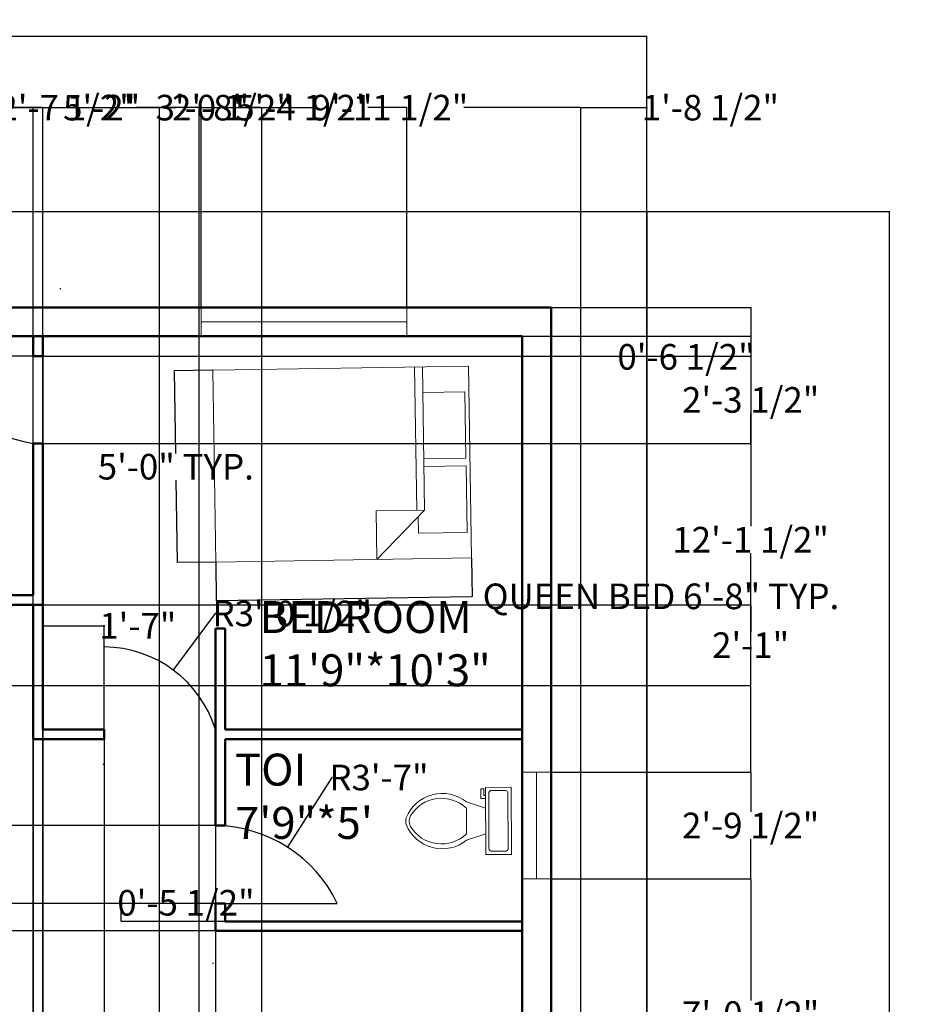
# Model space of a CAD drawing. Units: inches. Extents: x 3437 to 3994, y 3379 to 4084.
# Tile 6 of 6: x 3715 to 3994, y 3776 to 4084. Entities that reach past the tile are written whole.
import ezdxf

# ---------------------------------------------------------------- set-up
doc = ezdxf.new("R2010")
doc.units = ezdxf.units.IN
doc.header["$MEASUREMENT"] = 0
for name, color, linetype, lineweight in [('A-ANNO-DIMS', 2, 'Continuous', 18), ('A-AREA-IDEN', 7, 'Continuous', 25), ('A-DOOR', 3, 'Continuous', 25), ('A-FLOR-FIXT', 9, 'Continuous', 18), ('A-FURN', 8, 'Continuous', 18), ('A-GLAZ', 4, 'Continuous', 18), ('A-WALL', 7, 'Continuous', 50), ('C-PROP', 3, 'Continuous', 25)]:
    doc.layers.add(name, color=color, linetype=linetype, lineweight=lineweight)
doc.styles.get("Standard").update_dxf_attribs({"font": 'arial.ttf'})
doc.dimstyles.get("Standard").update_dxf_attribs({"dimtxt": 8, "dimasz": 0.18, "dimexe": 0.18, "dimexo": 0.0625, "dimgap": 0.09, "dimtad": 0, "dimtih": 1, "dimtoh": 1, "dimdec": 0, "dimzin": 0, "dimdsep": 46, "dimlunit": 3, "dimtxsty": 'Standard', "dimcen": 0.09, "dimadec": 0, "dimazin": 0, "dimtfac": 1, "dimtdec": 0, "dimtofl": 0, "dimtmove": 0, "dimatfit": 3, "dimfxl": 1, "dimtolj": 1, "dimtzin": 0, "dimarcsym": 0})

# ---------------------------------------------------------------- blocks, each defined once
blk = doc.blocks.new('Bed - Queen')
for p, q in [((0, -80.00003), (0, 0)), ((0, 0), (59.99999, 0)), ((59.99999, 0), (59.99999, -80.00003)), ((7.99999, -1.2), (28.79998, -1.2)), ((7.99999, -14.4), (7.99999, -1.2)), ((28.79998, -1.2), (28.79998, -14.4)), ((31.19999, -1.2), (51.99999, -1.2)), ((31.19999, -14.4), (31.19999, -1.2)), ((51.99999, -1.2), (51.99999, -16.4)), ((0, -14.4), (44.8, -14.4)), ((59.99999, -29.6), (44.8, -14.4)), ((44.8, -14.4), (44.8, -29.6)), ((44.8, -16.8), (0, -16.8)), ((51.99999, -16.4), (46.79936, -16.4)), ((44.8, -29.6), (59.99999, -29.6)), ((59.99999, -80.00003), (0, -80.00003))]:
    blk.add_line(p, q)
blk = doc.blocks.new('Toilet - top')
for p, q in [((9.5, -6), (9.5, -2)), ((-10, -8.5), (-8, -8.5)), ((-10, -9.5), (-10, -8.5)), ((-8, -8.5), (-8, -8)), ((-7, -8), (-7, -9.5)), ((-4, -8), (-6, -14)), ((4, -8), (6, -14)), ((-7, -9.5), (-10, -9.5)), ((4, -14), (-4, -14))]:
    blk.add_line(p, q)
blk.add_lwpolyline([(10.5, -8), (10.5, 0), (-10.5, 0), (-10.5, -8)], close=True)
for points in [[(-9.5, -2), (-9.5, -6)], [(8.5, -1), (-8.5, -1)], [(-8.5, -7), (8.5, -7)]]:
    blk.add_lwpolyline(points)
for centre, radius, start, end in [((-8.62, -1.88), 0.884, 81.8699, 188.1301), ((8.62, -1.88), 0.884, 351.8699, 98.1301), ((-8.62, -6.12), 0.884, 171.8699, 278.1301), ((8.62, -6.12), 0.884, 261.8699, 8.1301), ((3.52, -21.58), 12.17, 141.4691, 247.9714), ((4.2, -21.82), 11.33, 136.3677, 238.9468), ((-3.52, -21.58), 12.17, 292.0284, 38.5307), ((-4.2, -21.82), 11.33, 301.053, 43.6321), ((0, -27.88), 4, 245.7318, 294.2682), ((0, -29), 4, 254.8605, 285.1395)]:
    blk.add_arc(centre, radius, start, end)
blk = doc.blocks.new('*D9')
at = {"layer": 'A-ANNO-DIMS', "color": 0, "lineweight": -2, "transparency": 16777216}
for p, q in [((3491.02, 4023.7), (3491.02, 4078.52)), ((3491.2, 4078.34), (3694.15, 4078.34)), ((3910.84, 4078.34), (3707.9, 4078.34)), ((3911.02, 4023.7), (3911.02, 4078.52))]:
    blk.add_line(p, q, dxfattribs=at)
at = {"layer": 'A-ANNO-DIMS', "color": 0, "transparency": 16777216}
for points in [[(3491.2, 4078.37), (3491.2, 4078.31), (3491.02, 4078.34)], [(3910.84, 4078.37), (3910.84, 4078.31), (3911.02, 4078.34)]]:
    blk.add_solid(points, dxfattribs=at)
at = {"layer": 'Defpoints', "color": 0, "transparency": 16777216}
for p in [(3911.02, 4078.34), (3491.02, 4023.64), (3911.02, 4023.64)]:
    blk.add_point(p, dxfattribs=at)
at = {"layer": 'A-ANNO-DIMS', "color": 0, "transparency": 16777216, "insert": (3701.02, 4078.34), "char_height": 8, "attachment_point": 5}
blk.add_mtext("\\A1;35'", dxfattribs=at)
blk = doc.blocks.new('*D10')
at = {"layer": 'A-ANNO-DIMS', "color": 0, "lineweight": -2, "transparency": 16777216}
for p, q in [((3911.09, 4023.64), (3986.96, 4023.64)), ((3986.78, 4023.46), (3986.78, 3727.81)), ((3986.78, 3423.82), (3986.78, 3719.46)), ((3911.09, 3423.64), (3986.96, 3423.64))]:
    blk.add_line(p, q, dxfattribs=at)
at = {"layer": 'A-ANNO-DIMS', "color": 0, "transparency": 16777216}
for points in [[(3986.75, 4023.46), (3986.81, 4023.46), (3986.78, 4023.64)], [(3986.75, 3423.82), (3986.81, 3423.82), (3986.78, 3423.64)]]:
    blk.add_solid(points, dxfattribs=at)
at = {"layer": 'Defpoints', "color": 0, "transparency": 16777216}
for p in [(3911.02, 4023.64), (3986.78, 4023.64), (3911.02, 3423.64)]:
    blk.add_point(p, dxfattribs=at)
at = {"layer": 'A-ANNO-DIMS', "color": 0, "transparency": 16777216, "insert": (3986.78, 3723.64), "char_height": 8, "attachment_point": 5}
blk.add_mtext("\\A1;50'", dxfattribs=at)
blk = doc.blocks.new('*D13')
at = {"layer": 'A-ANNO-DIMS', "color": 0, "lineweight": -2, "transparency": 16777216}
for p, q in [((3776.11, 3913.95), (3776.3, 3901.83)), ((3856.1, 3915.21), (3856.29, 3903.1)), ((3776.48, 3902.01), (3856.11, 3903.27)), ((3856.29, 3903.28), (3856.47, 3903.28))]:
    blk.add_line(p, q, dxfattribs=at)
at = {"layer": 'A-ANNO-DIMS', "color": 0, "transparency": 16777216}
for points in [[(3776.48, 3902.04), (3776.48, 3901.98), (3776.3, 3902.01)], [(3856.11, 3903.3), (3856.11, 3903.24), (3856.29, 3903.28)]]:
    blk.add_solid(points, dxfattribs=at)
at = {"layer": 'Defpoints', "color": 0, "transparency": 16777216}
for p in [(3776.11, 3914.01), (3856.1, 3915.28), (3856.29, 3903.28)]:
    blk.add_point(p, dxfattribs=at)
at = {"layer": 'A-ANNO-DIMS', "color": 0, "transparency": 16777216, "insert": (3915.4, 3903.28), "char_height": 8, "attachment_point": 5}
blk.add_mtext('\\A1;QUEEN BED 6\'-8" TYP.', dxfattribs=at)
blk = doc.blocks.new('*D14')
at = {"layer": 'A-ANNO-DIMS', "color": 0, "lineweight": -2, "transparency": 16777216}
for p, q in [((3775.1, 3974), (3762.98, 3973.81)), ((3763.16, 3973.63), (3763.57, 3947.99)), ((3764.11, 3914), (3763.7, 3939.64)), ((3776.05, 3914.01), (3763.93, 3913.82))]:
    blk.add_line(p, q, dxfattribs=at)
at = {"layer": 'A-ANNO-DIMS', "color": 0, "transparency": 16777216}
for points in [[(3763.19, 3973.63), (3763.13, 3973.63), (3763.16, 3973.81)], [(3764.14, 3914), (3764.08, 3914), (3764.11, 3913.82)]]:
    blk.add_solid(points, dxfattribs=at)
at = {"layer": 'Defpoints', "color": 0, "transparency": 16777216}
for p in [(3775.16, 3974), (3764.11, 3913.82), (3776.11, 3914.01)]:
    blk.add_point(p, dxfattribs=at)
at = {"layer": 'A-ANNO-DIMS', "color": 0, "transparency": 16777216, "insert": (3763.63, 3943.81), "char_height": 8, "attachment_point": 5}
blk.add_mtext('\\A1;5\'-0" TYP.', dxfattribs=at)
blk = doc.blocks.new('*D32')
at = {"layer": 'A-ANNO-DIMS', "color": 0, "lineweight": -2, "transparency": 16777216}
for p, q in [((3678.02, 3993.7), (3678.02, 4056.27)), ((3678.2, 4056.09), (3709.13, 4056.09)), ((3709.31, 3993.7), (3709.31, 4056.27)), ((3709.31, 4056.09), (3709.49, 4056.09))]:
    blk.add_line(p, q, dxfattribs=at)
at = {"layer": 'A-ANNO-DIMS', "color": 0, "transparency": 16777216}
for points in [[(3678.2, 4056.12), (3678.2, 4056.06), (3678.02, 4056.09)], [(3709.13, 4056.12), (3709.13, 4056.06), (3709.31, 4056.09)]]:
    blk.add_solid(points, dxfattribs=at)
at = {"layer": 'Defpoints', "color": 0, "transparency": 16777216}
for p in [(3709.31, 4056.09), (3678.02, 3993.64), (3709.31, 3993.64)]:
    blk.add_point(p, dxfattribs=at)
at = {"layer": 'A-ANNO-DIMS', "color": 0, "transparency": 16777216, "insert": (3729.6, 4056.09), "char_height": 8, "attachment_point": 5}
blk.add_mtext('\\A1;2\'-7 1/2"', dxfattribs=at)
blk = doc.blocks.new('*D33')
at = {"layer": 'A-ANNO-DIMS', "color": 0, "lineweight": -2, "transparency": 16777216}
for p, q in [((3709.31, 3993.7), (3709.31, 4056.27)), ((3709.49, 4056.09), (3729.7, 4056.09)), ((3771.35, 4056.09), (3751.14, 4056.09)), ((3771.53, 3993.7), (3771.53, 4056.27))]:
    blk.add_line(p, q, dxfattribs=at)
at = {"layer": 'A-ANNO-DIMS', "color": 0, "transparency": 16777216}
for points in [[(3709.49, 4056.12), (3709.49, 4056.06), (3709.31, 4056.09)], [(3771.35, 4056.12), (3771.35, 4056.06), (3771.53, 4056.09)]]:
    blk.add_solid(points, dxfattribs=at)
at = {"layer": 'Defpoints', "color": 0, "transparency": 16777216}
for p in [(3771.53, 4056.09), (3709.31, 3993.64), (3771.53, 3993.64)]:
    blk.add_point(p, dxfattribs=at)
at = {"layer": 'A-ANNO-DIMS', "color": 0, "transparency": 16777216, "insert": (3740.42, 4056.09), "char_height": 8, "attachment_point": 5}
blk.add_mtext('\\A1;5\'-2"', dxfattribs=at)
blk = doc.blocks.new('*D34')
at = {"layer": 'A-ANNO-DIMS', "color": 0, "lineweight": -2, "transparency": 16777216}
for p, q in [((3771.53, 3993.7), (3771.53, 4056.27)), ((3771.71, 4056.09), (3783.65, 4056.09)), ((3835.68, 4056.09), (3823.74, 4056.09)), ((3835.86, 3993.7), (3835.86, 4056.27))]:
    blk.add_line(p, q, dxfattribs=at)
at = {"layer": 'A-ANNO-DIMS', "color": 0, "transparency": 16777216}
for points in [[(3771.71, 4056.12), (3771.71, 4056.06), (3771.53, 4056.09)], [(3835.68, 4056.12), (3835.68, 4056.06), (3835.86, 4056.09)]]:
    blk.add_solid(points, dxfattribs=at)
at = {"layer": 'Defpoints', "color": 0, "transparency": 16777216}
for p in [(3835.86, 4056.09), (3771.53, 3993.64), (3835.86, 3993.64)]:
    blk.add_point(p, dxfattribs=at)
at = {"layer": 'A-ANNO-DIMS', "color": 0, "transparency": 16777216, "insert": (3803.69, 4056.09), "char_height": 8, "attachment_point": 5}
blk.add_mtext('\\A1;5\'-4 1/2"', dxfattribs=at)
blk = doc.blocks.new('*D41')
at = {"layer": 'A-ANNO-DIMS', "color": 0, "lineweight": -2, "transparency": 16777216}
for p, q in [((3881.09, 3993.64), (3943.65, 3993.64)), ((3943.47, 3993.46), (3943.47, 3925.2)), ((3943.47, 3848.5), (3943.47, 3916.75)), ((3881.09, 3848.32), (3943.65, 3848.32))]:
    blk.add_line(p, q, dxfattribs=at)
at = {"layer": 'A-ANNO-DIMS', "color": 0, "transparency": 16777216}
for points in [[(3943.44, 3993.46), (3943.5, 3993.46), (3943.47, 3993.64)], [(3943.44, 3848.5), (3943.5, 3848.5), (3943.47, 3848.32)]]:
    blk.add_solid(points, dxfattribs=at)
at = {"layer": 'Defpoints', "color": 0, "transparency": 16777216}
for p in [(3881.02, 3993.64), (3881.02, 3848.32), (3943.47, 3848.32)]:
    blk.add_point(p, dxfattribs=at)
at = {"layer": 'A-ANNO-DIMS', "color": 0, "transparency": 16777216, "insert": (3943.47, 3920.98), "char_height": 8, "attachment_point": 5}
blk.add_mtext('\\A1;12\'-1 1/2"', dxfattribs=at)
blk = doc.blocks.new('*D42')
at = {"layer": 'A-ANNO-DIMS', "color": 0, "lineweight": -2, "transparency": 16777216}
for p, q in [((3881.09, 3848.32), (3943.65, 3848.32)), ((3943.47, 3848.14), (3943.47, 3835.85)), ((3943.47, 3815.1), (3943.47, 3827.39)), ((3881.09, 3814.92), (3943.65, 3814.92))]:
    blk.add_line(p, q, dxfattribs=at)
at = {"layer": 'A-ANNO-DIMS', "color": 0, "transparency": 16777216}
for points in [[(3943.44, 3848.14), (3943.5, 3848.14), (3943.47, 3848.32)], [(3943.44, 3815.1), (3943.5, 3815.1), (3943.47, 3814.92)]]:
    blk.add_solid(points, dxfattribs=at)
at = {"layer": 'Defpoints', "color": 0, "transparency": 16777216}
for p in [(3881.02, 3848.32), (3881.02, 3814.92), (3943.47, 3814.92)]:
    blk.add_point(p, dxfattribs=at)
at = {"layer": 'A-ANNO-DIMS', "color": 0, "transparency": 16777216, "insert": (3943.47, 3831.62), "char_height": 8, "attachment_point": 5}
blk.add_mtext('\\A1;2\'-9 1/2"', dxfattribs=at)
blk = doc.blocks.new('*D43')
at = {"layer": 'A-ANNO-DIMS', "color": 0, "lineweight": -2, "transparency": 16777216}
for p, q in [((3881.09, 3814.92), (3943.65, 3814.92)), ((3943.47, 3814.74), (3943.47, 3776.88)), ((3943.47, 3730.56), (3943.47, 3768.42)), ((3881.09, 3730.38), (3943.65, 3730.38))]:
    blk.add_line(p, q, dxfattribs=at)
at = {"layer": 'A-ANNO-DIMS', "color": 0, "transparency": 16777216}
for points in [[(3943.44, 3814.74), (3943.5, 3814.74), (3943.47, 3814.92)], [(3943.44, 3730.56), (3943.5, 3730.56), (3943.47, 3730.38)]]:
    blk.add_solid(points, dxfattribs=at)
at = {"layer": 'Defpoints', "color": 0, "transparency": 16777216}
for p in [(3881.02, 3814.92), (3881.02, 3730.38), (3943.47, 3730.38)]:
    blk.add_point(p, dxfattribs=at)
at = {"layer": 'A-ANNO-DIMS', "color": 0, "transparency": 16777216, "insert": (3943.47, 3772.65), "char_height": 8, "attachment_point": 5}
blk.add_mtext('\\A1;7\'-0 1/2"', dxfattribs=at)
blk = doc.blocks.new('*D46')
at = {"layer": 'A-ANNO-DIMS', "color": 0, "lineweight": -2, "transparency": 16777216}
for p, q in [((3576.02, 3426.7), (3576.02, 4056.27)), ((3576.2, 4056.09), (3635.57, 4056.09)), ((3721.84, 4056.09), (3662.48, 4056.09)), ((3722.02, 3426.7), (3722.02, 4056.27))]:
    blk.add_line(p, q, dxfattribs=at)
at = {"layer": 'A-ANNO-DIMS', "color": 0, "transparency": 16777216}
for points in [[(3576.2, 4056.12), (3576.2, 4056.06), (3576.02, 4056.09)], [(3721.84, 4056.12), (3721.84, 4056.06), (3722.02, 4056.09)]]:
    blk.add_solid(points, dxfattribs=at)
at = {"layer": 'Defpoints', "color": 0, "transparency": 16777216}
for p in [(3722.02, 4056.09), (3576.02, 3426.64), (3722.02, 3426.64)]:
    blk.add_point(p, dxfattribs=at)
at = {"layer": 'A-ANNO-DIMS', "color": 0, "transparency": 16777216, "insert": (3649.02, 4056.09), "char_height": 8, "attachment_point": 5}
blk.add_mtext('\\A1;12\'-2"', dxfattribs=at)
blk = doc.blocks.new('*D48')
at = {"layer": 'A-ANNO-DIMS', "color": 0, "lineweight": -2, "transparency": 16777216}
for p, q in [((3722.02, 3861.57), (3722.02, 3391.01)), ((3719.02, 3858.57), (3719.02, 3391.01)), ((3719.2, 3391.19), (3721.84, 3391.19)), ((3722.02, 3391.19), (3722.2, 3391.19))]:
    blk.add_line(p, q, dxfattribs=at)
at = {"layer": 'A-ANNO-DIMS', "color": 0, "transparency": 16777216}
for points in [[(3719.2, 3391.22), (3719.2, 3391.16), (3719.02, 3391.19)], [(3721.84, 3391.22), (3721.84, 3391.16), (3722.02, 3391.19)]]:
    blk.add_solid(points, dxfattribs=at)
at = {"layer": 'Defpoints', "color": 0, "transparency": 16777216}
for p in [(3722.02, 3861.64), (3719.02, 3858.64), (3722.02, 3391.19)]:
    blk.add_point(p, dxfattribs=at)
at = {"layer": 'A-ANNO-DIMS', "color": 0, "transparency": 16777216, "insert": (3732.93, 3391.19), "char_height": 8, "attachment_point": 5}
blk.add_mtext('\\A1;0\'-3"', dxfattribs=at)
blk = doc.blocks.new('*D49')
at = {"layer": 'A-ANNO-DIMS', "color": 0, "lineweight": -2, "transparency": 16777216}
for p, q in [((3530.02, 3504.7), (3530.02, 4056.27)), ((3530.2, 4056.09), (3611.07, 4056.09)), ((3718.84, 4056.09), (3637.98, 4056.09)), ((3719.02, 3504.7), (3719.02, 4056.27))]:
    blk.add_line(p, q, dxfattribs=at)
at = {"layer": 'A-ANNO-DIMS', "color": 0, "transparency": 16777216}
for points in [[(3530.2, 4056.12), (3530.2, 4056.06), (3530.02, 4056.09)], [(3718.84, 4056.12), (3718.84, 4056.06), (3719.02, 4056.09)]]:
    blk.add_solid(points, dxfattribs=at)
at = {"layer": 'Defpoints', "color": 0, "transparency": 16777216}
for p in [(3719.02, 4056.09), (3530.02, 3504.64), (3719.02, 3504.64)]:
    blk.add_point(p, dxfattribs=at)
at = {"layer": 'A-ANNO-DIMS', "color": 0, "transparency": 16777216, "insert": (3624.52, 4056.09), "char_height": 8, "attachment_point": 5}
blk.add_mtext('\\A1;15\'-9"', dxfattribs=at)
blk = doc.blocks.new('*D53')
at = {"layer": 'A-ANNO-DIMS', "color": 0, "lineweight": -2, "transparency": 16777216}
for p, q in [((3770.9, 3426.7), (3770.9, 4056.27)), ((3771.08, 4056.09), (3807.48, 4056.09)), ((3890.18, 4056.09), (3853.78, 4056.09)), ((3890.36, 3426.7), (3890.36, 4056.27))]:
    blk.add_line(p, q, dxfattribs=at)
at = {"layer": 'A-ANNO-DIMS', "color": 0, "transparency": 16777216}
for points in [[(3771.08, 4056.12), (3771.08, 4056.06), (3770.9, 4056.09)], [(3890.18, 4056.12), (3890.18, 4056.06), (3890.36, 4056.09)]]:
    blk.add_solid(points, dxfattribs=at)
at = {"layer": 'Defpoints', "color": 0, "transparency": 16777216}
for p in [(3890.36, 4056.09), (3770.9, 3426.64), (3890.36, 3426.64)]:
    blk.add_point(p, dxfattribs=at)
at = {"layer": 'A-ANNO-DIMS', "color": 0, "transparency": 16777216, "insert": (3830.63, 4056.09), "char_height": 8, "attachment_point": 5}
blk.add_mtext('\\A1;9\'-11 1/2"', dxfattribs=at)
blk = doc.blocks.new('*D54')
at = {"layer": 'A-ANNO-DIMS', "color": 0, "lineweight": -2, "transparency": 16777216}
for p, q in [((3890.36, 3426.7), (3890.36, 4056.27)), ((3890.54, 4056.09), (3910.84, 4056.09)), ((3911.02, 3426.7), (3911.02, 4056.27)), ((3911.02, 4056.09), (3911.2, 4056.09))]:
    blk.add_line(p, q, dxfattribs=at)
at = {"layer": 'A-ANNO-DIMS', "color": 0, "transparency": 16777216}
for points in [[(3890.54, 4056.12), (3890.54, 4056.06), (3890.36, 4056.09)], [(3910.84, 4056.12), (3910.84, 4056.06), (3911.02, 4056.09)]]:
    blk.add_solid(points, dxfattribs=at)
at = {"layer": 'Defpoints', "color": 0, "transparency": 16777216}
for p in [(3911.02, 4056.09), (3890.36, 3426.64), (3911.02, 3426.64)]:
    blk.add_point(p, dxfattribs=at)
at = {"layer": 'A-ANNO-DIMS', "color": 0, "transparency": 16777216, "insert": (3930.87, 4056.09), "char_height": 8, "attachment_point": 5}
blk.add_mtext('\\A1;1\'-8 1/2"', dxfattribs=at)
blk = doc.blocks.new('*D55')
at = {"layer": 'A-ANNO-DIMS', "color": 0, "lineweight": -2, "transparency": 16777216}
for p, q in [((3662.09, 3900.64), (3943.65, 3900.64)), ((3943.47, 3900.46), (3943.47, 3892.12)), ((3943.47, 3875.57), (3943.47, 3883.91)), ((3662.09, 3875.39), (3943.65, 3875.39))]:
    blk.add_line(p, q, dxfattribs=at)
at = {"layer": 'A-ANNO-DIMS', "color": 0, "transparency": 16777216}
for points in [[(3943.44, 3900.46), (3943.5, 3900.46), (3943.47, 3900.64)], [(3943.44, 3875.57), (3943.5, 3875.57), (3943.47, 3875.39)]]:
    blk.add_solid(points, dxfattribs=at)
at = {"layer": 'Defpoints', "color": 0, "transparency": 16777216}
for p in [(3662.02, 3900.64), (3662.02, 3875.39), (3943.47, 3875.39)]:
    blk.add_point(p, dxfattribs=at)
at = {"layer": 'A-ANNO-DIMS', "color": 0, "transparency": 16777216, "insert": (3943.47, 3888.01), "char_height": 8, "attachment_point": 5}
blk.add_mtext('\\A1;2\'-1"', dxfattribs=at)
blk = doc.blocks.new('*D56')
at = {"layer": 'A-ANNO-DIMS', "color": 0, "lineweight": -2, "transparency": 16777216}
for p, q in [((3719.09, 3978.34), (3943.65, 3978.34)), ((3943.47, 3978.16), (3943.47, 3968.92)), ((3943.47, 3951.22), (3943.47, 3960.46)), ((3719.09, 3951.04), (3943.65, 3951.04))]:
    blk.add_line(p, q, dxfattribs=at)
at = {"layer": 'A-ANNO-DIMS', "color": 0, "transparency": 16777216}
for points in [[(3943.44, 3978.16), (3943.5, 3978.16), (3943.47, 3978.34)], [(3943.44, 3951.22), (3943.5, 3951.22), (3943.47, 3951.04)]]:
    blk.add_solid(points, dxfattribs=at)
at = {"layer": 'Defpoints', "color": 0, "transparency": 16777216}
for p in [(3719.02, 3978.34), (3719.02, 3951.04), (3943.47, 3951.04)]:
    blk.add_point(p, dxfattribs=at)
at = {"layer": 'A-ANNO-DIMS', "color": 0, "transparency": 16777216, "insert": (3943.47, 3964.69), "char_height": 8, "attachment_point": 5}
blk.add_mtext('\\A1;2\'-3 1/2"', dxfattribs=at)
blk = doc.blocks.new('*D57')
at = {"layer": 'A-ANNO-DIMS', "color": 0, "lineweight": -2, "transparency": 16777216}
for p, q in [((3741.22, 3861.57), (3741.22, 3391.01)), ((3776.02, 3861.57), (3776.02, 3391.01)), ((3741.4, 3391.19), (3744.72, 3391.19)), ((3775.84, 3391.19), (3772.52, 3391.19))]:
    blk.add_line(p, q, dxfattribs=at)
at = {"layer": 'A-ANNO-DIMS', "color": 0, "transparency": 16777216}
for points in [[(3741.4, 3391.22), (3741.4, 3391.16), (3741.22, 3391.19)], [(3775.84, 3391.22), (3775.84, 3391.16), (3776.02, 3391.19)]]:
    blk.add_solid(points, dxfattribs=at)
at = {"layer": 'Defpoints', "color": 0, "transparency": 16777216}
for p in [(3741.22, 3861.64), (3776.02, 3861.64), (3776.02, 3391.19)]:
    blk.add_point(p, dxfattribs=at)
at = {"layer": 'A-ANNO-DIMS', "color": 0, "transparency": 16777216, "insert": (3758.62, 3391.19), "char_height": 8, "attachment_point": 5}
blk.add_mtext('\\A1;2\'-11"', dxfattribs=at)
blk = doc.blocks.new('*D58')
at = {"layer": 'A-ANNO-DIMS', "color": 0, "lineweight": -2, "transparency": 16777216}
for p, q in [((3775.96, 3831.64), (3458.39, 3831.64)), ((3458.57, 3831.46), (3458.57, 3823.68)), ((3458.57, 3807.45), (3458.57, 3815.23)), ((3775.96, 3807.27), (3458.39, 3807.27))]:
    blk.add_line(p, q, dxfattribs=at)
at = {"layer": 'A-ANNO-DIMS', "color": 0, "transparency": 16777216}
for points in [[(3458.54, 3831.46), (3458.6, 3831.46), (3458.57, 3831.64)], [(3458.54, 3807.45), (3458.6, 3807.45), (3458.57, 3807.27)]]:
    blk.add_solid(points, dxfattribs=at)
at = {"layer": 'Defpoints', "color": 0, "transparency": 16777216}
for p in [(3776.02, 3831.64), (3458.57, 3807.27), (3776.02, 3807.27)]:
    blk.add_point(p, dxfattribs=at)
at = {"layer": 'A-ANNO-DIMS', "color": 0, "transparency": 16777216, "insert": (3458.57, 3819.45), "char_height": 8, "attachment_point": 5}
blk.add_mtext('\\A1;2\'-0 1/2"', dxfattribs=at)
blk = doc.blocks.new('*D64')
at = {"layer": 'A-ANNO-DIMS', "color": 0, "lineweight": -2, "transparency": 16777216}
for p, q in [((3722.02, 3718.27), (3722.02, 4056.27)), ((3722.2, 4056.09), (3758.36, 4056.09)), ((3758.54, 3718.27), (3758.54, 4056.27)), ((3758.54, 4056.09), (3758.72, 4056.09))]:
    blk.add_line(p, q, dxfattribs=at)
at = {"layer": 'A-ANNO-DIMS', "color": 0, "transparency": 16777216}
for points in [[(3722.2, 4056.12), (3722.2, 4056.06), (3722.02, 4056.09)], [(3758.36, 4056.12), (3758.36, 4056.06), (3758.54, 4056.09)]]:
    blk.add_solid(points, dxfattribs=at)
at = {"layer": 'Defpoints', "color": 0, "transparency": 16777216}
for p in [(3758.54, 4056.09), (3722.02, 3718.21), (3758.54, 3718.21)]:
    blk.add_point(p, dxfattribs=at)
at = {"layer": 'A-ANNO-DIMS', "color": 0, "transparency": 16777216, "insert": (3778.76, 4056.09), "char_height": 8, "attachment_point": 5}
blk.add_mtext('\\A1;3\'-0 1/2"', dxfattribs=at)
blk = doc.blocks.new('*D71')
at = {"layer": 'A-ANNO-DIMS', "color": 0, "lineweight": -2, "transparency": 16777216}
for p, q in [((3719.09, 3984.64), (3943.65, 3984.64)), ((3943.47, 3984.46), (3943.47, 3978.52)), ((3719.09, 3978.34), (3943.65, 3978.34)), ((3943.47, 3978.16), (3943.29, 3978.16)), ((3943.47, 3978.34), (3943.47, 3978.16))]:
    blk.add_line(p, q, dxfattribs=at)
at = {"layer": 'A-ANNO-DIMS', "color": 0, "transparency": 16777216}
for points in [[(3943.44, 3984.46), (3943.5, 3984.46), (3943.47, 3984.64)], [(3943.44, 3978.52), (3943.5, 3978.52), (3943.47, 3978.34)]]:
    blk.add_solid(points, dxfattribs=at)
at = {"layer": 'Defpoints', "color": 0, "transparency": 16777216}
for p in [(3719.02, 3984.64), (3719.02, 3978.34), (3943.47, 3978.34)]:
    blk.add_point(p, dxfattribs=at)
at = {"layer": 'A-ANNO-DIMS', "color": 0, "transparency": 16777216, "insert": (3923.25, 3978.16), "char_height": 8, "attachment_point": 5}
blk.add_mtext('\\A1;0\'-6 1/2"', dxfattribs=at)
blk = doc.blocks.new('*D72')
at = {"layer": 'A-ANNO-DIMS', "color": 0, "lineweight": -2, "transparency": 16777216}
for p, q in [((3722.02, 3861.7), (3722.02, 3894.27)), ((3722.2, 3894.09), (3741.04, 3894.09)), ((3741.22, 3861.7), (3741.22, 3894.27)), ((3741.22, 3894.09), (3741.4, 3894.09))]:
    blk.add_line(p, q, dxfattribs=at)
at = {"layer": 'A-ANNO-DIMS', "color": 0, "transparency": 16777216}
for points in [[(3722.2, 3894.12), (3722.2, 3894.06), (3722.02, 3894.09)], [(3741.04, 3894.12), (3741.04, 3894.06), (3741.22, 3894.09)]]:
    blk.add_solid(points, dxfattribs=at)
at = {"layer": 'Defpoints', "color": 0, "transparency": 16777216}
for p in [(3741.22, 3894.09), (3722.02, 3861.64), (3741.22, 3861.64)]:
    blk.add_point(p, dxfattribs=at)
at = {"layer": 'A-ANNO-DIMS', "color": 0, "transparency": 16777216, "insert": (3751.74, 3894.09), "char_height": 8, "attachment_point": 5}
blk.add_mtext('\\A1;1\'-7"', dxfattribs=at)
blk = doc.blocks.new('*D78')
at = {"layer": 'A-ANNO-DIMS', "color": 0, "lineweight": -2, "transparency": 16777216}
for p, q in [((3778.96, 3807.27), (3746.39, 3807.27)), ((3746.57, 3807.27), (3746.57, 3807.45)), ((3746.57, 3807.45), (3746.75, 3807.45)), ((3746.57, 3801.82), (3746.57, 3807.09)), ((3778.96, 3801.64), (3746.39, 3801.64))]:
    blk.add_line(p, q, dxfattribs=at)
at = {"layer": 'A-ANNO-DIMS', "color": 0, "transparency": 16777216}
for points in [[(3746.54, 3807.09), (3746.6, 3807.09), (3746.57, 3807.27)], [(3746.54, 3801.82), (3746.6, 3801.82), (3746.57, 3801.64)]]:
    blk.add_solid(points, dxfattribs=at)
at = {"layer": 'Defpoints', "color": 0, "transparency": 16777216}
for p in [(3746.57, 3807.27), (3779.02, 3807.27), (3779.02, 3801.64)]:
    blk.add_point(p, dxfattribs=at)
at = {"layer": 'A-ANNO-DIMS', "color": 0, "transparency": 16777216, "insert": (3766.8, 3807.45), "char_height": 8, "attachment_point": 5}
blk.add_mtext('\\A1;0\'-5 1/2"', dxfattribs=at)
blk = doc.blocks.new('*D79')
at = {"layer": 'A-ANNO-DIMS', "color": 0, "lineweight": -2, "transparency": 16777216}
for p, q in [((3675.76, 3905.25), (3675.76, 3391.01)), ((3665.02, 3903.57), (3665.02, 3391.01)), ((3665.2, 3391.19), (3675.58, 3391.19)), ((3675.76, 3391.19), (3675.94, 3391.19))]:
    blk.add_line(p, q, dxfattribs=at)
at = {"layer": 'A-ANNO-DIMS', "color": 0, "transparency": 16777216}
for points in [[(3665.2, 3391.22), (3665.2, 3391.16), (3665.02, 3391.19)], [(3675.58, 3391.22), (3675.58, 3391.16), (3675.76, 3391.19)]]:
    blk.add_solid(points, dxfattribs=at)
at = {"layer": 'Defpoints', "color": 0, "transparency": 16777216}
for p in [(3675.76, 3905.31), (3665.02, 3903.64), (3675.76, 3391.19)]:
    blk.add_point(p, dxfattribs=at)
at = {"layer": 'A-ANNO-DIMS', "color": 0, "transparency": 16777216, "insert": (3699.09, 3391.19), "char_height": 8, "attachment_point": 5}
blk.add_mtext('\\A1;0\'-10 1/2"', dxfattribs=at)
blk = doc.blocks.new('*D81')
at = {"layer": 'A-ANNO-DIMS', "color": 0, "lineweight": -2, "transparency": 16777216}
for p, q in [((3722.02, 3984.57), (3722.02, 3391.01)), ((3872.02, 3984.57), (3872.02, 3391.01)), ((3722.2, 3391.19), (3783.57, 3391.19)), ((3871.84, 3391.19), (3810.48, 3391.19))]:
    blk.add_line(p, q, dxfattribs=at)
at = {"layer": 'A-ANNO-DIMS', "color": 0, "transparency": 16777216}
for points in [[(3722.2, 3391.22), (3722.2, 3391.16), (3722.02, 3391.19)], [(3871.84, 3391.22), (3871.84, 3391.16), (3872.02, 3391.19)]]:
    blk.add_solid(points, dxfattribs=at)
at = {"layer": 'Defpoints', "color": 0, "transparency": 16777216}
for p in [(3722.02, 3984.64), (3872.02, 3984.64), (3872.02, 3391.19)]:
    blk.add_point(p, dxfattribs=at)
at = {"layer": 'A-ANNO-DIMS', "color": 0, "transparency": 16777216, "insert": (3797.02, 3391.19), "char_height": 8, "attachment_point": 5}
blk.add_mtext('\\A1;12\'-6"', dxfattribs=at)
blk = doc.blocks.new('*D83')
at = {"layer": 'A-ANNO-DIMS', "color": 0, "lineweight": -2, "transparency": 16777216}
for p, q in [((3758.54, 3667.46), (3758.54, 4056.27)), ((3758.72, 4056.09), (3763.72, 4056.09)), ((3790.31, 4056.09), (3785.3, 4056.09)), ((3790.49, 3664.77), (3790.49, 4056.27))]:
    blk.add_line(p, q, dxfattribs=at)
at = {"layer": 'A-ANNO-DIMS', "color": 0, "transparency": 16777216}
for points in [[(3758.72, 4056.12), (3758.72, 4056.06), (3758.54, 4056.09)], [(3790.31, 4056.12), (3790.31, 4056.06), (3790.49, 4056.09)]]:
    blk.add_solid(points, dxfattribs=at)
at = {"layer": 'Defpoints', "color": 0, "transparency": 16777216}
for p in [(3790.49, 4056.09), (3758.54, 3667.39), (3790.49, 3664.71)]:
    blk.add_point(p, dxfattribs=at)
at = {"layer": 'A-ANNO-DIMS', "color": 0, "transparency": 16777216, "insert": (3774.51, 4056.09), "char_height": 8, "attachment_point": 5}
blk.add_mtext('\\A1;2\'-8"', dxfattribs=at)
blk = doc.blocks.new('*D86')
at = {"layer": 'A-ANNO-DIMS', "color": 0, "lineweight": -2, "transparency": 16777216}
for p, q in [((3775.96, 3798.64), (3458.39, 3798.64)), ((3458.57, 3798.46), (3458.57, 3786.05)), ((3458.57, 3765.19), (3458.57, 3777.6)), ((3791.17, 3765.01), (3458.39, 3765.01))]:
    blk.add_line(p, q, dxfattribs=at)
at = {"layer": 'A-ANNO-DIMS', "color": 0, "transparency": 16777216}
for points in [[(3458.54, 3798.46), (3458.6, 3798.46), (3458.57, 3798.64)], [(3458.54, 3765.19), (3458.6, 3765.19), (3458.57, 3765.01)]]:
    blk.add_solid(points, dxfattribs=at)
at = {"layer": 'Defpoints', "color": 0, "transparency": 16777216}
for p in [(3776.02, 3798.64), (3458.57, 3765.01), (3791.23, 3765.01)]:
    blk.add_point(p, dxfattribs=at)
at = {"layer": 'A-ANNO-DIMS', "color": 0, "transparency": 16777216, "insert": (3458.57, 3781.82), "char_height": 8, "attachment_point": 5}
blk.add_mtext('\\A1;2\'-9 1/2"', dxfattribs=at)
blk = doc.blocks.new('*D90')
at = {"layer": 'A-ANNO-DIMS', "color": 0, "lineweight": -2, "transparency": 16777216}
for p, q in [((3812.45, 3846.62), (3798.63, 3825.01)), ((3812.63, 3846.62), (3812.45, 3846.62)), ((3775.26, 3788.59), (3775.44, 3788.59)), ((3775.35, 3788.5), (3775.35, 3788.68))]:
    blk.add_line(p, q, dxfattribs=at)
at = {"layer": 'A-ANNO-DIMS', "color": 0, "transparency": 16777216}
blk.add_solid([(3798.61, 3825.03), (3798.66, 3825), (3798.54, 3824.86)], dxfattribs=at)
at = {"layer": 'Defpoints', "color": 0, "transparency": 16777216}
for p in [(3798.54, 3824.86), (3775.35, 3788.59)]:
    blk.add_point(p, dxfattribs=at)
at = {"layer": 'A-ANNO-DIMS', "color": 0, "transparency": 16777216, "insert": (3827.18, 3846.62), "char_height": 8, "attachment_point": 5}
blk.add_mtext('\\A1;R3\'-7"', dxfattribs=at)
blk = doc.blocks.new('*D92')
at = {"layer": 'A-ANNO-DIMS', "color": 0, "lineweight": -2, "transparency": 16777216}
for p, q in [((3775.96, 3897.92), (3762.95, 3880.39)), ((3776.14, 3897.92), (3775.96, 3897.92)), ((3740.88, 3850.77), (3741.06, 3850.77)), ((3740.97, 3850.68), (3740.97, 3850.86))]:
    blk.add_line(p, q, dxfattribs=at)
at = {"layer": 'A-ANNO-DIMS', "color": 0, "transparency": 16777216}
blk.add_solid([(3762.93, 3880.4), (3762.97, 3880.37), (3762.84, 3880.24)], dxfattribs=at)
at = {"layer": 'Defpoints', "color": 0, "transparency": 16777216}
for p in [(3762.84, 3880.24), (3740.97, 3850.77)]:
    blk.add_point(p, dxfattribs=at)
at = {"layer": 'A-ANNO-DIMS', "color": 0, "transparency": 16777216, "insert": (3800.02, 3897.92), "char_height": 8, "attachment_point": 5}
blk.add_mtext('\\A1;R3\'-0 1/2"', dxfattribs=at)
blk = doc.blocks.new('*D95')
at = {"layer": 'A-ANNO-DIMS', "color": 0, "lineweight": -2, "transparency": 16777216}
for p, q in [((3727.49, 3999.57), (3727.67, 3999.57)), ((3727.58, 3999.48), (3727.58, 3999.66)), ((3670.64, 3945.04), (3691.86, 3965.37)), ((3670.46, 3945.04), (3670.64, 3945.04))]:
    blk.add_line(p, q, dxfattribs=at)
at = {"layer": 'A-ANNO-DIMS', "color": 0, "transparency": 16777216}
blk.add_solid([(3691.84, 3965.39), (3691.88, 3965.34), (3691.99, 3965.49)], dxfattribs=at)
at = {"layer": 'Defpoints', "color": 0, "transparency": 16777216}
for p in [(3727.58, 3999.57), (3691.99, 3965.49)]:
    blk.add_point(p, dxfattribs=at)
at = {"layer": 'A-ANNO-DIMS', "color": 0, "transparency": 16777216, "insert": (3646.59, 3945.04), "char_height": 8, "attachment_point": 5}
blk.add_mtext('\\A1;R4\'-1 1/2"', dxfattribs=at)

msp = doc.modelspace()

# ---------------------------------------------------------------- linework, layer by layer
at = {"layer": 'A-DOOR'}
for p, q in [((3719.02, 3978.34), (3683.11, 3978.34)), ((3741.22, 3861.64), (3741.22, 3887.47)), ((3779.02, 3807.27), (3814.13, 3807.27))]:
    msp.add_line(p, q, dxfattribs=at)
for centre, radius, start, end in [((3727.58, 3999.57), 49.27, 205.5271, 260.0037), ((3740.97, 3850.77), 36.7, 17.2182, 89.6185), ((3775.35, 3788.59), 43.05, 25.7132, 89.0985)]:
    msp.add_arc(centre, radius, start, end, dxfattribs=at)
at = {"layer": 'A-GLAZ'}
for p, q in [((3771.53, 3993.64), (3771.53, 3984.64)), ((3835.86, 3993.64), (3835.86, 3984.64)), ((3771.53, 3989.14), (3835.86, 3989.14)), ((3872.02, 3848.32), (3881.02, 3848.32)), ((3876.52, 3848.32), (3876.52, 3814.92)), ((3872.02, 3814.92), (3881.02, 3814.92))]:
    msp.add_line(p, q, dxfattribs=at)
at = {"layer": 'A-WALL'}
for p, q in [((3521.02, 3993.64), (3881.02, 3993.64)), ((3881.02, 3993.64), (3881.02, 3618.64)), ((3665.02, 3984.64), (3872.02, 3984.64)), ((3719.02, 3978.34), (3719.02, 3984.64)), ((3722.02, 3978.34), (3722.02, 3984.64)), ((3872.02, 3984.64), (3872.02, 3621.64)), ((3719.02, 3978.34), (3722.02, 3978.34)), ((3719.02, 3903.64), (3719.02, 3951.04)), ((3719.02, 3951.04), (3722.02, 3951.04)), ((3722.02, 3861.64), (3722.02, 3951.04)), ((3665.02, 3903.64), (3719.02, 3903.64)), ((3665.02, 3900.64), (3722.02, 3900.64)), ((3719.02, 3858.64), (3719.02, 3900.64)), ((3776.02, 3861.64), (3776.02, 3893.27)), ((3776.02, 3893.27), (3779.02, 3893.27)), ((3779.02, 3893.27), (3779.02, 3861.64)), ((3722.02, 3861.64), (3741.22, 3861.64)), ((3741.22, 3861.64), (3741.22, 3858.64)), ((3776.02, 3861.64), (3776.02, 3831.64)), ((3779.02, 3861.64), (3872.02, 3861.64)), ((3722.02, 3858.64), (3719.02, 3858.64)), ((3722.02, 3858.64), (3741.22, 3858.64)), ((3779.02, 3858.64), (3779.02, 3831.64)), ((3779.02, 3858.64), (3872.02, 3858.64)), ((3776.02, 3831.64), (3779.02, 3831.64)), ((3776.02, 3807.27), (3779.02, 3807.27)), ((3776.02, 3807.27), (3776.02, 3801.64)), ((3779.02, 3807.27), (3779.02, 3801.64)), ((3776.02, 3801.64), (3776.02, 3798.64)), ((3779.02, 3801.64), (3872.02, 3801.64)), ((3776.02, 3798.64), (3872.02, 3798.64))]:
    msp.add_line(p, q, dxfattribs=at)
at = {"layer": 'C-PROP'}
msp.add_line((3911.02, 4023.64), (3911.02, 3426.64), dxfattribs=at)
msp.add_lwpolyline([(3770.9, 3423.64), (3491.02, 3423.64), (3491.02, 4023.64), (3911.02, 4023.64), (3911.02, 3423.64), (3890.36, 3423.64)], dxfattribs=at)

# ---------------------------------------------------------------- block references
at = {"layer": 'A-FLOR-FIXT', "rotation": 270.2194248225682}
msp.add_blockref('Toilet - top', (3868.56, 3833.08), dxfattribs=at)
at = {"layer": 'A-FURN', "rotation": 270.90745513795}
msp.add_blockref('Bed - Queen', (3855.15, 3975.27), dxfattribs=at)

# ---------------------------------------------------------------- texts
at = {"layer": 'A-AREA-IDEN', "char_height": 10, "attachment_point": 1}
for s, insert in [('BEDROOM\\P11\'9"*10\'3"', (3789.85, 3901.81)), ('TOI\\P7\'9"*5\'', (3782.16, 3854.09))]:
    msp.add_mtext_dynamic_manual_height_columns(s, width=200.853, gutter_width=1, heights=[0], dxfattribs=dict(at, insert=insert))

# ---------------------------------------------------------------- dimensions: what is measured, and where the dimension line sits
at = {"layer": 'A-ANNO-DIMS'}
for base, p1, p2, override, picture, middle in [((3911.02, 4078.34), (3491.02, 4023.64), (3911.02, 4023.64), {"dimclrd": 0, "dimclre": 0, "dimclrt": 0}, '*D9', (3701.02, 4078.34)), ((3709.31, 4056.09), (3678.02, 3993.64), (3709.31, 3993.64), {"dimdec": 1, "dimlfac": 1, "dimrnd": 0, "dimzin": 1, "dimdsep": 46, "dimlunit": 4, "dimfrac": 2}, '*D32', (3729.6, 4056.09)), ((3758.54, 4056.09), (3722.02, 3718.21), (3758.54, 3718.21), {"dimdec": 1, "dimlfac": 1, "dimrnd": 0, "dimzin": 1, "dimdsep": 46, "dimlunit": 4, "dimfrac": 2}, '*D64', (3778.76, 4056.09)), ((3890.36, 4056.09), (3770.9, 3426.64), (3890.36, 3426.64), {"dimdec": 1, "dimlfac": 1, "dimrnd": 0, "dimzin": 1, "dimdsep": 46, "dimlunit": 4, "dimfrac": 2}, '*D53', (3830.63, 4056.09)), ((3835.86, 4056.09), (3771.53, 3993.64), (3835.86, 3993.64), {"dimdec": 1, "dimlfac": 1, "dimrnd": 0, "dimzin": 1, "dimdsep": 46, "dimlunit": 4, "dimfrac": 2}, '*D34', (3803.69, 4056.09)), ((3911.02, 4056.09), (3890.36, 3426.64), (3911.02, 3426.64), {"dimdec": 1, "dimlfac": 1, "dimrnd": 0, "dimzin": 1, "dimdsep": 46, "dimlunit": 4, "dimfrac": 2}, '*D54', (3930.87, 4056.09)), ((3719.02, 4056.09), (3530.02, 3504.64), (3719.02, 3504.64), {"dimdec": 1, "dimlfac": 1, "dimrnd": 0, "dimzin": 1, "dimdsep": 46, "dimlunit": 4, "dimfrac": 2}, '*D49', (3624.52, 4056.09)), ((3722.02, 4056.09), (3576.02, 3426.64), (3722.02, 3426.64), {"dimdec": 1, "dimlfac": 1, "dimrnd": 0, "dimzin": 1, "dimdsep": 46, "dimlunit": 4, "dimfrac": 2}, '*D46', (3649.02, 4056.09)), ((3771.53, 4056.09), (3709.31, 3993.64), (3771.53, 3993.64), {"dimdec": 1, "dimlfac": 1, "dimrnd": 0, "dimzin": 1, "dimdsep": 46, "dimlunit": 4, "dimfrac": 2}, '*D33', (3740.42, 4056.09)), ((3790.4858, 4056.0859), (3758.54, 3667.394), (3790.4858, 3664.706), {"dimdec": 1, "dimlfac": 1, "dimrnd": 0, "dimzin": 1, "dimdsep": 46, "dimlunit": 4, "dimfrac": 2}, '*D83', (3774.5129, 4056.0859)), ((3872.02, 3391.19), (3722.02, 3984.64), (3872.02, 3984.64), {"dimdec": 1, "dimlfac": 1, "dimrnd": 0, "dimzin": 1, "dimdsep": 46, "dimlunit": 4, "dimfrac": 2}, '*D81', (3797.02, 3391.19)), ((3675.76, 3391.19), (3665.02, 3903.64), (3675.76, 3905.31), {"dimdec": 1, "dimlfac": 1, "dimrnd": 0, "dimzin": 1, "dimdsep": 46, "dimlunit": 4, "dimfrac": 2}, '*D79', (3699.09, 3391.19)), ((3741.22, 3894.09), (3722.02, 3861.64), (3741.22, 3861.64), {"dimdec": 1, "dimlfac": 1, "dimrnd": 0, "dimzin": 1, "dimdsep": 46, "dimlunit": 4, "dimfrac": 2}, '*D72', (3751.74, 3894.09)), ((3722.02, 3391.19), (3719.02, 3858.64), (3722.02, 3861.64), {"dimdec": 1, "dimlfac": 1, "dimrnd": 0, "dimzin": 1, "dimdsep": 46, "dimlunit": 4, "dimfrac": 2}, '*D48', (3732.93, 3391.19)), ((3776.02, 3391.19), (3741.22, 3861.64), (3776.02, 3861.64), {"dimdec": 1, "dimlfac": 1, "dimrnd": 0, "dimzin": 1, "dimdsep": 46, "dimlunit": 4, "dimfrac": 2}, '*D57', (3758.62, 3391.19))]:
    dim = msp.add_linear_dim(base=base, p1=p1, p2=p2, dimstyle='Standard', override=override, dxfattribs=at)
    dim.commit()
    dim.dimension.update_dxf_attribs({"geometry": picture, "text_midpoint": middle})
for base, p1, p2, override, picture, middle in [((3986.78, 4023.64), (3911.02, 3423.64), (3911.02, 4023.64), {"dimclrd": 0, "dimclre": 0, "dimclrt": 0}, '*D10', (3986.78, 3723.64)), ((3943.47, 3848.32), (3881.02, 3993.64), (3881.02, 3848.32), {"dimdec": 1, "dimlfac": 1, "dimrnd": 0, "dimzin": 1, "dimdsep": 46, "dimlunit": 4, "dimfrac": 2}, '*D41', (3943.47, 3920.98)), ((3943.47, 3978.34), (3719.02, 3984.64), (3719.02, 3978.34), {"dimdec": 1, "dimlfac": 1, "dimrnd": 0, "dimzin": 1, "dimdsep": 46, "dimlunit": 4, "dimfrac": 2}, '*D71', (3923.25, 3978.16)), ((3943.47, 3951.04), (3719.02, 3978.34), (3719.02, 3951.04), {"dimdec": 1, "dimlfac": 1, "dimrnd": 0, "dimzin": 1, "dimdsep": 46, "dimlunit": 4, "dimfrac": 2}, '*D56', (3943.47, 3964.69)), ((3943.4743, 3875.389), (3662.0243, 3900.6359), (3662.0243, 3875.389), {"dimdec": 1, "dimlfac": 1, "dimrnd": 0, "dimzin": 1, "dimdsep": 46, "dimlunit": 4, "dimfrac": 2}, '*D55', (3943.4743, 3888.0125)), ((3943.47, 3814.92), (3881.02, 3848.32), (3881.02, 3814.92), {"dimdec": 1, "dimlfac": 1, "dimrnd": 0, "dimzin": 1, "dimdsep": 46, "dimlunit": 4, "dimfrac": 2}, '*D42', (3943.47, 3831.62)), ((3458.57, 3807.27), (3776.02, 3831.64), (3776.02, 3807.27), {"dimdec": 1, "dimlfac": 1, "dimrnd": 0, "dimzin": 1, "dimdsep": 46, "dimlunit": 4, "dimfrac": 2}, '*D58', (3458.57, 3819.45)), ((3746.57, 3807.27), (3779.02, 3801.64), (3779.02, 3807.27), {"dimdec": 1, "dimlfac": 1, "dimrnd": 0, "dimzin": 1, "dimdsep": 46, "dimlunit": 4, "dimfrac": 2}, '*D78', (3766.8, 3807.45)), ((3943.47, 3730.38), (3881.02, 3814.92), (3881.02, 3730.38), {"dimdec": 1, "dimlfac": 1, "dimrnd": 0, "dimzin": 1, "dimdsep": 46, "dimlunit": 4, "dimfrac": 2}, '*D43', (3943.47, 3772.65)), ((3458.57, 3765.01), (3776.02, 3798.64), (3791.23, 3765.01), {"dimdec": 1, "dimlfac": 1, "dimrnd": 0, "dimzin": 1, "dimdsep": 46, "dimlunit": 4, "dimfrac": 2}, '*D86', (3458.57, 3781.82))]:
    dim = msp.add_linear_dim(base=base, p1=p1, p2=p2, angle=90, dimstyle='Standard', override=override, dxfattribs=at)
    dim.commit()
    dim.dimension.update_dxf_attribs({"geometry": picture, "text_midpoint": middle})
for center, mpoint, picture, middle in [((3727.58, 3999.57), (3691.99, 3965.49), '*D95', (3646.59, 3945.04)), ((3740.97, 3850.77), (3762.84, 3880.24), '*D92', (3800.02, 3897.92)), ((3775.347, 3788.591), (3798.5379, 3824.8609), '*D90', (3827.1836, 3846.6228))]:
    dim = msp.add_radius_dim(center=center, mpoint=mpoint, dimstyle='Standard', override={"dimdec": 1, "dimlfac": 1, "dimrnd": 0, "dimzin": 1, "dimdsep": 46, "dimlunit": 4, "dimfrac": 2}, dxfattribs=at)
    dim.commit()
    dim.dimension.update_dxf_attribs({"geometry": picture, "text_midpoint": middle, "dimtype": 164})
for base, p1, p2, angle, text, picture, middle in [((3764.11, 3913.82), (3775.16, 3974), (3776.11, 3914.01), 270.9075, '<> TYP.', '*D14', (3763.63, 3943.81)), ((3856.29, 3903.28), (3776.11, 3914.01), (3856.1, 3915.28), 0.9075, 'QUEEN BED <> TYP.', '*D13', (3915.4, 3903.28))]:
    dim = msp.add_linear_dim(base=base, p1=p1, p2=p2, angle=angle, text=text, dimstyle='Standard', override={"dimdec": 1, "dimlfac": 1, "dimrnd": 0, "dimzin": 1, "dimdsep": 46, "dimlunit": 4, "dimfrac": 2}, dxfattribs=at)
    dim.commit()
    dim.dimension.update_dxf_attribs({"geometry": picture, "text_midpoint": middle})

doc.saveas('drawing.dxf')
